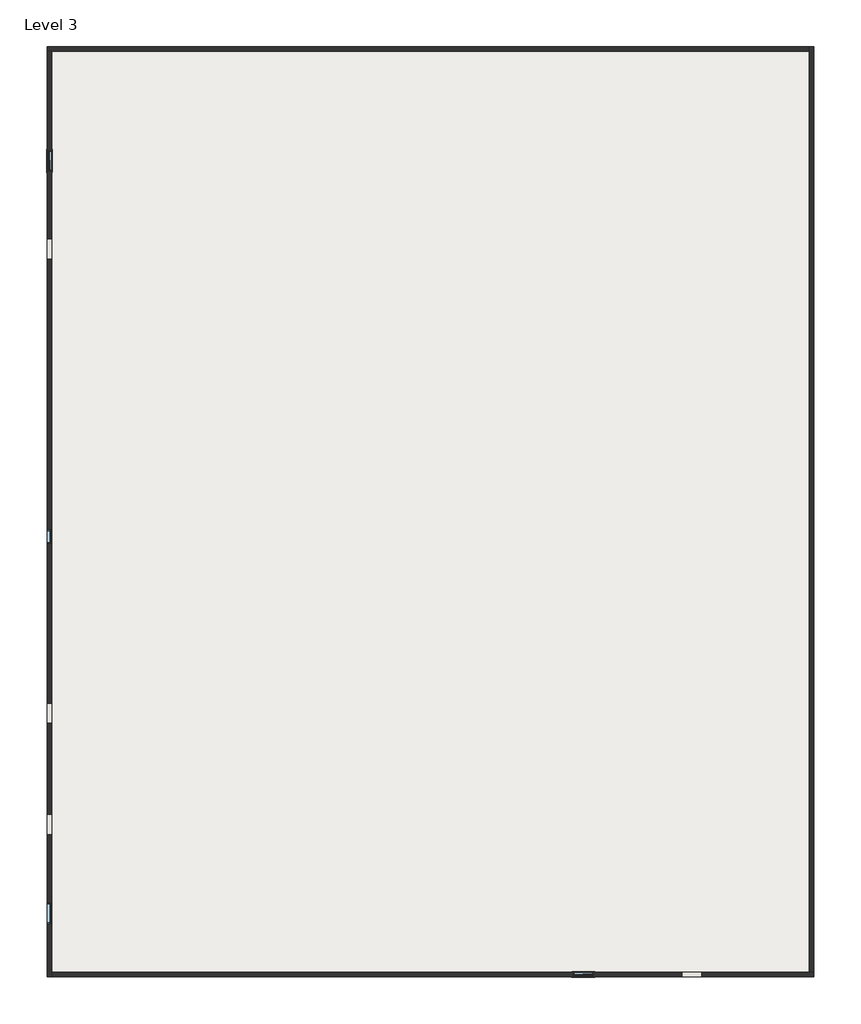
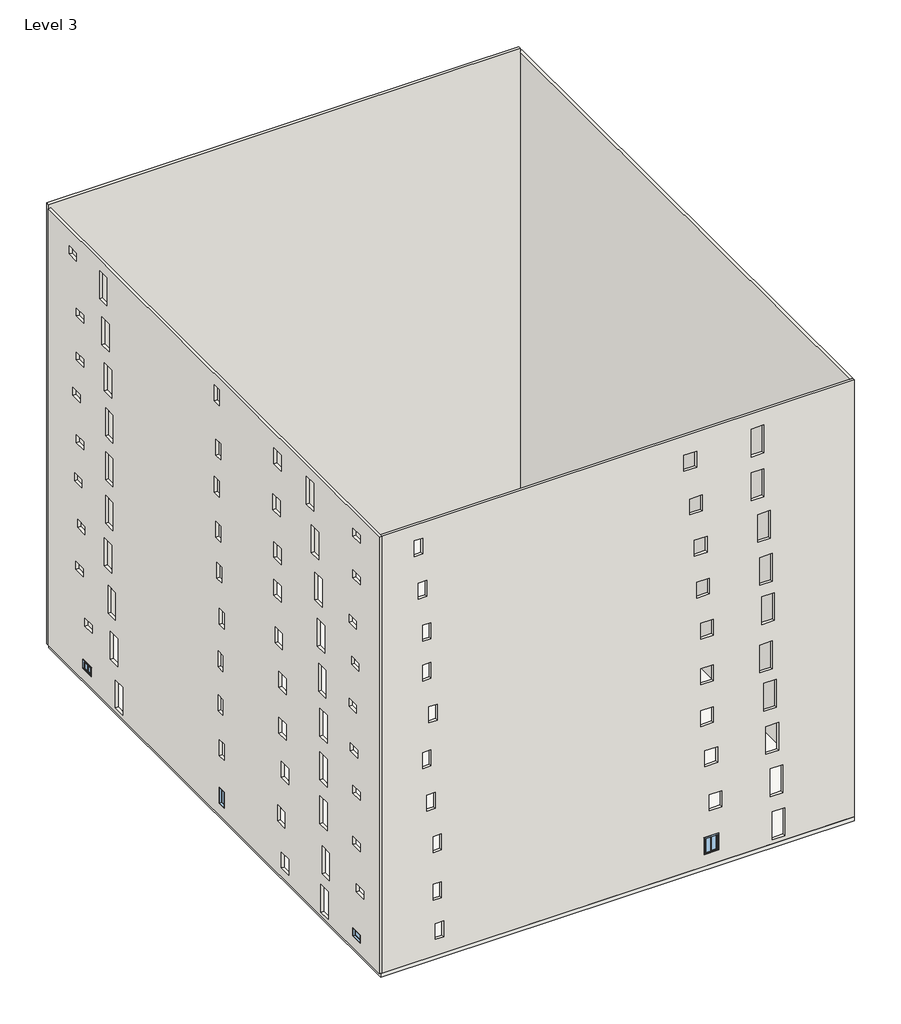
# One storey: 4 walls, 4 windows, 1 slab.
"""IFC4 building model written with IfcOpenShell, lengths in millimetres."""

from ifc_helpers import new_model, si_unit, frame, origin, place, context, project, spatial, polyline, outline, extrude, faceted_brep, transform, mapped, element, save
from components import window_80bd9af0, window_57c3ee1c, window_a4355bb3, window_54100e87

model = new_model("IFC4")

# Units and contexts
model_context = context("Model", 3, world=origin())
ifc_project = project(units=[si_unit("LENGTHUNIT", "METRE", prefix="MILLI")], contexts=[model_context])

# Site, building, storey
site = spatial("IfcSite", under=ifc_project)
building = spatial("IfcBuilding", under=site)
storey = spatial("IfcBuildingStorey", under=building, Name="Level 3", Elevation=6096.0)

# Slab
placement = place(None, origin())
element("IfcSlab", 1, ObjectType="Generic - 12\"", at=placement, inside=storey, context=model_context, shape_type="SweptSolid", body=[
    extrude(outline(polyline([(19165.761926, 20810.2014639), (19165.761926, -20845.7985361), (-15175.038074, -20845.7985361), (-15175.038074, 20810.2014639), (19165.761926, 20810.2014639)])), frame((0.0, 0.0, 5791.2), z_axis=(0.0, 0.0, 1.0), x_axis=(1.0, 0.0, 0.0)), (0.0, 0.0, 1.0), 304.8),
])

# Walls
element("IfcWall", 2, ObjectType="Generic - 8\"", at=placement, inside=storey, context=model_context, shape_type="Brep", body=[
    faceted_brep([(-15276.638074, 20708.6014639, 6096.0), (-15073.438074, 20708.6014639, 6096.0), (18962.561926, 20708.6014639, 6096.0), (18962.561926, 20708.6014639, 39865.082979), (-15276.638074, 20708.6014639, 39865.082979), (-15276.638074, 20708.6014639, 39560.282979), (-15276.638074, 20911.8014639, 6096.0), (-15276.638074, 20911.8014639, 39865.082979), (18962.561926, 20911.8014639, 39865.082979), (18962.561926, 20911.8014639, 39560.282979), (18962.561926, 20911.8014639, 6096.0)], [[[0, 1, 2, 3, 4, 5]], [[6, 7, 8, 9, 10]], [[2, 1, 0, 6, 10]], [[4, 3, 8, 7]], [[0, 5, 4, 7, 6]], [[3, 2, 10, 9, 8]]]),
])
element("IfcWall", 3, ObjectType="Generic - 8\"", at=placement, inside=storey, context=model_context, shape_type="Brep", body=[
    faceted_brep([(-15073.438074, -20845.7985361, 6096.0), (-15073.438074, -20642.5985361, 6096.0), (-15073.438074, 20708.6014639, 6096.0), (-15073.438074, 20708.6014639, 39560.282979), (-15073.438074, -20642.5985361, 39560.282979), (-15073.438074, -20845.7985361, 39560.282979), (-15073.438074, 13342.6014639, 36576.0), (-15073.438074, 13342.6014639, 38709.6), (-15073.438074, 14257.0014639, 38709.6), (-15073.438074, 14257.0014639, 36576.0), (-15073.438074, 13037.8014639, 33223.2), (-15073.438074, 13037.8014639, 35356.8), (-15073.438074, 13952.2014639, 35356.8), (-15073.438074, 13952.2014639, 33223.2), (-15073.438074, 12733.0014639, 29870.4), (-15073.438074, 12733.0014639, 32004.0), (-15073.438074, 13647.4014639, 32004.0), (-15073.438074, 13647.4014639, 29870.4), (-15073.438074, 12580.6014639, 26517.6), (-15073.438074, 12580.6014639, 28651.2), (-15073.438074, 13495.0014639, 28651.2), (-15073.438074, 13495.0014639, 26517.6), (-15073.438074, 12580.6014639, 23164.8), (-15073.438074, 12580.6014639, 25298.4), (-15073.438074, 13495.0014639, 25298.4), (-15073.438074, 13495.0014639, 23164.8), (-15073.438074, 12580.6014639, 19812.0), (-15073.438074, 12580.6014639, 21945.6), (-15073.438074, 13495.0014639, 21945.6), (-15073.438074, 13495.0014639, 19812.0), (-15073.438074, 12733.0014639, 16459.2), (-15073.438074, 12733.0014639, 18592.8), (-15073.438074, 13647.4014639, 18592.8), (-15073.438074, 13647.4014639, 16459.2), (-15073.438074, 12275.8014639, 13106.4), (-15073.438074, 12275.8014639, 15240.0), (-15073.438074, 13190.2014639, 15240.0), (-15073.438074, 13190.2014639, 13106.4), (-15073.438074, 11971.0014639, 9753.6), (-15073.438074, 11971.0014639, 11887.2), (-15073.438074, 12885.4014639, 11887.2), (-15073.438074, 12885.4014639, 9753.6), (-15073.438074, 11361.4014639, 6400.8), (-15073.438074, 11361.4014639, 8534.4), (-15073.438074, 12275.8014639, 8534.4), (-15073.438074, 12275.8014639, 6400.8), (-15073.438074, -12633.3915889, 36576.0), (-15073.438074, -12633.3915889, 38709.6), (-15073.438074, -11718.9915889, 38709.6), (-15073.438074, -11718.9915889, 36576.0), (-15073.438074, -13242.9915889, 33223.2), (-15073.438074, -13242.9915889, 35356.8), (-15073.438074, -12328.5915889, 35356.8), (-15073.438074, -12328.5915889, 33223.2), (-15073.438074, -13700.1915889, 29870.4), (-15073.438074, -13700.1915889, 32004.0), (-15073.438074, -12785.7915889, 32004.0), (-15073.438074, -12785.7915889, 29870.4), (-15073.438074, -14004.9915889, 26517.6), (-15073.438074, -14004.9915889, 28651.2), (-15073.438074, -13090.5915889, 28651.2), (-15073.438074, -13090.5915889, 26517.6), (-15073.438074, -14157.3915889, 23164.8), (-15073.438074, -14157.3915889, 25298.4), (-15073.438074, -13242.9915889, 25298.4), (-15073.438074, -13242.9915889, 23164.8), (-15073.438074, -14309.7915889, 19812.0), (-15073.438074, -14309.7915889, 21945.6), (-15073.438074, -13395.3915889, 21945.6), (-15073.438074, -13395.3915889, 19812.0), (-15073.438074, -14309.7915889, 16459.2), (-15073.438074, -14309.7915889, 18592.8), (-15073.438074, -13395.3915889, 18592.8), (-15073.438074, -13395.3915889, 16459.2), (-15073.438074, -14309.7915889, 13106.4), (-15073.438074, -14309.7915889, 15240.0), (-15073.438074, -13395.3915889, 15240.0), (-15073.438074, -13395.3915889, 13106.4), (-15073.438074, -14462.1915889, 6400.8), (-15073.438074, -14462.1915889, 8534.4), (-15073.438074, -13547.7915889, 8534.4), (-15073.438074, -13547.7915889, 6400.8), (-15073.438074, -14614.5915889, 9448.8), (-15073.438074, -14614.5915889, 11582.4), (-15073.438074, -13700.1915889, 11582.4), (-15073.438074, -13700.1915889, 9448.8), (-15073.438074, -7643.2213044, 38404.8), (-15073.438074, -7643.2213044, 37185.6), (-15073.438074, -8557.6213044, 37185.6), (-15073.438074, -8557.6213044, 38404.8), (-15073.438074, -7490.8213044, 34807.3666062), (-15073.438074, -7490.8213044, 33588.1666062), (-15073.438074, -8405.2213044, 33588.1666062), (-15073.438074, -8405.2213044, 34807.3666062), (-15073.438074, -7617.8213044, 31211.5058376), (-15073.438074, -7617.8213044, 29992.3058376), (-15073.438074, -8532.2213044, 29992.3058376), (-15073.438074, -8532.2213044, 31211.5058376), (-15073.438074, -7643.2213044, 28346.4), (-15073.438074, -7643.2213044, 27127.2), (-15073.438074, -8557.6213044, 27127.2), (-15073.438074, -8557.6213044, 28346.4), (-15073.438074, -7795.6213044, 24794.8201055), (-15073.438074, -7795.6213044, 23575.6201055), (-15073.438074, -8710.0213044, 23575.6201055), (-15073.438074, -8710.0213044, 24794.8201055), (-15073.438074, -8252.8213044, 21640.8), (-15073.438074, -8252.8213044, 20421.6), (-15073.438074, -9167.2213044, 20421.6), (-15073.438074, -9167.2213044, 21640.8), (-15073.438074, -8252.8213044, 18137.3013379), (-15073.438074, -8252.8213044, 16918.1013379), (-15073.438074, -9167.2213044, 16918.1013379), (-15073.438074, -9167.2213044, 18137.3013379), (-15073.438074, -8557.6213044, 14935.2), (-15073.438074, -8557.6213044, 13716.0), (-15073.438074, -9472.0213044, 13716.0), (-15073.438074, -9472.0213044, 14935.2), (-15073.438074, -8100.4213044, 11325.7414578), (-15073.438074, -8100.4213044, 10106.5414578), (-15073.438074, -9014.8213044, 10106.5414578), (-15073.438074, -9014.8213044, 11325.7414578), (-15073.438074, -8557.6213044, 7986.372861), (-15073.438074, -8557.6213044, 6767.172861), (-15073.438074, -9472.0213044, 6767.172861), (-15073.438074, -9472.0213044, 7986.372861), (-15073.438074, -785.2213044, 38709.6), (-15073.438074, -175.6213044, 38709.6), (-15073.438074, -175.6213044, 37490.4), (-15073.438074, -785.2213044, 37490.4), (-15073.438074, -937.6213044, 34644.418592), (-15073.438074, -328.0213044, 34644.418592), (-15073.438074, -328.0213044, 33425.218592), (-15073.438074, -937.6213044, 33425.218592), (-15073.438074, -785.2213044, 31699.2), (-15073.438074, -175.6213044, 31699.2), (-15073.438074, -175.6213044, 30480.0), (-15073.438074, -785.2213044, 30480.0), (-15073.438074, -937.6213044, 28346.4), (-15073.438074, -328.0213044, 28346.4), (-15073.438074, -328.0213044, 27127.2), (-15073.438074, -937.6213044, 27127.2), (-15073.438074, -1090.0213044, 25298.4), (-15073.438074, -480.4213044, 25298.4), (-15073.438074, -480.4213044, 24079.2), (-15073.438074, -1090.0213044, 24079.2), (-15073.438074, -1394.8213044, 21945.6), (-15073.438074, -785.2213044, 21945.6), (-15073.438074, -785.2213044, 20726.4), (-15073.438074, -1394.8213044, 20726.4), (-15073.438074, -1242.4213044, 18592.8), (-15073.438074, -632.8213044, 18592.8), (-15073.438074, -632.8213044, 17373.6), (-15073.438074, -1242.4213044, 17373.6), (-15073.438074, -1242.4213044, 15240.0), (-15073.438074, -632.8213044, 15240.0), (-15073.438074, -632.8213044, 14020.8), (-15073.438074, -1242.4213044, 14020.8), (-15073.438074, -1394.8213044, 11887.2), (-15073.438074, -785.2213044, 11887.2), (-15073.438074, -785.2213044, 10668.0), (-15073.438074, -1394.8213044, 10668.0), (-15073.438074, -1394.8213044, 8229.6), (-15073.438074, -785.2213044, 8229.6), (-15073.438074, -785.2213044, 7010.4), (-15073.438074, -1394.8213044, 7010.4), (-15073.438074, 18067.0014639, 38292.0078244), (-15073.438074, 18067.0014639, 37682.4078244), (-15073.438074, 17152.6014639, 37682.4078244), (-15073.438074, 17152.6014639, 38292.0078244), (-15073.438074, 17152.6014639, 34092.765286), (-15073.438074, 17152.6014639, 33483.165286), (-15073.438074, 16238.2014639, 33483.165286), (-15073.438074, 16238.2014639, 34092.765286), (-15073.438074, 17152.6014639, 30718.6975007), (-15073.438074, 17152.6014639, 30109.0975007), (-15073.438074, 16238.2014639, 30109.0975007), (-15073.438074, 16238.2014639, 30718.6975007), (-15073.438074, 17609.8014639, 27736.8), (-15073.438074, 17609.8014639, 27127.2), (-15073.438074, 16695.4014639, 27127.2), (-15073.438074, 16695.4014639, 27736.8), (-15073.438074, 17152.6014639, 24384.0), (-15073.438074, 17152.6014639, 23774.4), (-15073.438074, 16238.2014639, 23774.4), (-15073.438074, 16238.2014639, 24384.0), (-15073.438074, 17381.2014639, 21336.0), (-15073.438074, 17381.2014639, 20726.4), (-15073.438074, 16466.8014639, 20726.4), (-15073.438074, 16466.8014639, 21336.0), (-15073.438074, 17000.2014639, 17983.2), (-15073.438074, 17000.2014639, 17373.6), (-15073.438074, 16085.8014639, 17373.6), (-15073.438074, 16085.8014639, 17983.2), (-15073.438074, 17228.8014639, 14630.4), (-15073.438074, 17228.8014639, 14020.8), (-15073.438074, 16314.4014639, 14020.8), (-15073.438074, 16314.4014639, 14630.4), (-15073.438074, 16085.8014639, 10972.8), (-15073.438074, 16085.8014639, 10363.2), (-15073.438074, 15171.4014639, 10363.2), (-15073.438074, 15171.4014639, 10972.8), (-15073.438074, 16238.2014639, 7620.0), (-15073.438074, 16238.2014639, 7010.4), (-15073.438074, 15323.8014639, 7010.4), (-15073.438074, 15323.8014639, 7620.0), (-15073.438074, -18460.9099202, 38259.9868241), (-15073.438074, -17546.5099202, 38259.9868241), (-15073.438074, -17546.5099202, 37650.3868241), (-15073.438074, -18460.9099202, 37650.3868241), (-15073.438074, -18460.9099202, 35069.665757), (-15073.438074, -17546.5099202, 35069.665757), (-15073.438074, -17546.5099202, 34460.065757), (-15073.438074, -18460.9099202, 34460.065757), (-15073.438074, -18006.4213044, 31394.4), (-15073.438074, -17092.0213044, 31394.4), (-15073.438074, -17092.0213044, 30784.8), (-15073.438074, -18006.4213044, 30784.8), (-15073.438074, -18311.2213044, 28348.6132762), (-15073.438074, -17396.8213044, 28348.6132762), (-15073.438074, -17396.8213044, 27739.0132762), (-15073.438074, -18311.2213044, 27739.0132762), (-15073.438074, -18006.4213044, 24953.0717638), (-15073.438074, -17092.0213044, 24953.0717638), (-15073.438074, -17092.0213044, 24343.4717638), (-15073.438074, -18006.4213044, 24343.4717638), (-15073.438074, -18158.8213044, 21626.4980928), (-15073.438074, -17244.4213044, 21626.4980928), (-15073.438074, -17244.4213044, 21016.8980928), (-15073.438074, -18158.8213044, 21016.8980928), (-15073.438074, -18460.9099202, 18571.6304295), (-15073.438074, -17546.5099202, 18571.6304295), (-15073.438074, -17546.5099202, 17962.0304295), (-15073.438074, -18460.9099202, 17962.0304295), (-15073.438074, -18460.9099202, 14630.4), (-15073.438074, -17546.5099202, 14630.4), (-15073.438074, -17546.5099202, 14020.8), (-15073.438074, -18460.9099202, 14020.8), (-15073.438074, -18915.3985361, 11277.6), (-15073.438074, -18000.9985361, 11277.6), (-15073.438074, -18000.9985361, 10668.0), (-15073.438074, -18915.3985361, 10668.0), (-15073.438074, -18460.9099202, 7620.0), (-15073.438074, -17546.5099202, 7620.0), (-15073.438074, -17546.5099202, 7010.4), (-15073.438074, -18460.9099202, 7010.4), (-15276.638074, -20845.7985361, 6096.0), (-15276.638074, -20845.7985361, 39560.282979), (-15276.638074, 20708.6014639, 39560.282979), (-15276.638074, 20708.6014639, 6096.0), (-15276.638074, 13342.6014639, 36576.0), (-15276.638074, 14257.0014639, 36576.0), (-15276.638074, 14257.0014639, 38709.6), (-15276.638074, 13342.6014639, 38709.6), (-15276.638074, 13037.8014639, 33223.2), (-15276.638074, 13952.2014639, 33223.2), (-15276.638074, 13952.2014639, 35356.8), (-15276.638074, 13037.8014639, 35356.8), (-15276.638074, 12733.0014639, 29870.4), (-15276.638074, 13647.4014639, 29870.4), (-15276.638074, 13647.4014639, 32004.0), (-15276.638074, 12733.0014639, 32004.0), (-15276.638074, 12580.6014639, 26517.6), (-15276.638074, 13495.0014639, 26517.6), (-15276.638074, 13495.0014639, 28651.2), (-15276.638074, 12580.6014639, 28651.2), (-15276.638074, 12580.6014639, 23164.8), (-15276.638074, 13495.0014639, 23164.8), (-15276.638074, 13495.0014639, 25298.4), (-15276.638074, 12580.6014639, 25298.4), (-15276.638074, 12580.6014639, 19812.0), (-15276.638074, 13495.0014639, 19812.0), (-15276.638074, 13495.0014639, 21945.6), (-15276.638074, 12580.6014639, 21945.6), (-15276.638074, 12733.0014639, 16459.2), (-15276.638074, 13647.4014639, 16459.2), (-15276.638074, 13647.4014639, 18592.8), (-15276.638074, 12733.0014639, 18592.8), (-15276.638074, 12275.8014639, 13106.4), (-15276.638074, 13190.2014639, 13106.4), (-15276.638074, 13190.2014639, 15240.0), (-15276.638074, 12275.8014639, 15240.0), (-15276.638074, 11971.0014639, 9753.6), (-15276.638074, 12885.4014639, 9753.6), (-15276.638074, 12885.4014639, 11887.2), (-15276.638074, 11971.0014639, 11887.2), (-15276.638074, 11361.4014639, 6400.8), (-15276.638074, 12275.8014639, 6400.8), (-15276.638074, 12275.8014639, 8534.4), (-15276.638074, 11361.4014639, 8534.4), (-15276.638074, -12633.3915889, 36576.0), (-15276.638074, -11718.9915889, 36576.0), (-15276.638074, -11718.9915889, 38709.6), (-15276.638074, -12633.3915889, 38709.6), (-15276.638074, -13242.9915889, 33223.2), (-15276.638074, -12328.5915889, 33223.2), (-15276.638074, -12328.5915889, 35356.8), (-15276.638074, -13242.9915889, 35356.8), (-15276.638074, -13700.1915889, 29870.4), (-15276.638074, -12785.7915889, 29870.4), (-15276.638074, -12785.7915889, 32004.0), (-15276.638074, -13700.1915889, 32004.0), (-15276.638074, -14004.9915889, 26517.6), (-15276.638074, -13090.5915889, 26517.6), (-15276.638074, -13090.5915889, 28651.2), (-15276.638074, -14004.9915889, 28651.2), (-15276.638074, -14157.3915889, 23164.8), (-15276.638074, -13242.9915889, 23164.8), (-15276.638074, -13242.9915889, 25298.4), (-15276.638074, -14157.3915889, 25298.4), (-15276.638074, -14309.7915889, 19812.0), (-15276.638074, -13395.3915889, 19812.0), (-15276.638074, -13395.3915889, 21945.6), (-15276.638074, -14309.7915889, 21945.6), (-15276.638074, -14309.7915889, 16459.2), (-15276.638074, -13395.3915889, 16459.2), (-15276.638074, -13395.3915889, 18592.8), (-15276.638074, -14309.7915889, 18592.8), (-15276.638074, -14309.7915889, 13106.4), (-15276.638074, -13395.3915889, 13106.4), (-15276.638074, -13395.3915889, 15240.0), (-15276.638074, -14309.7915889, 15240.0), (-15276.638074, -14462.1915889, 6400.8), (-15276.638074, -13547.7915889, 6400.8), (-15276.638074, -13547.7915889, 8534.4), (-15276.638074, -14462.1915889, 8534.4), (-15276.638074, -14614.5915889, 9448.8), (-15276.638074, -13700.1915889, 9448.8), (-15276.638074, -13700.1915889, 11582.4), (-15276.638074, -14614.5915889, 11582.4), (-15276.638074, -7643.2213044, 38404.8), (-15276.638074, -8557.6213044, 38404.8), (-15276.638074, -8557.6213044, 37185.6), (-15276.638074, -7643.2213044, 37185.6), (-15276.638074, -7490.8213044, 34807.3666062), (-15276.638074, -8405.2213044, 34807.3666062), (-15276.638074, -8405.2213044, 33588.1666062), (-15276.638074, -7490.8213044, 33588.1666062), (-15276.638074, -7617.8213044, 31211.5058376), (-15276.638074, -8532.2213044, 31211.5058376), (-15276.638074, -8532.2213044, 29992.3058376), (-15276.638074, -7617.8213044, 29992.3058376), (-15276.638074, -7643.2213044, 28346.4), (-15276.638074, -8557.6213044, 28346.4), (-15276.638074, -8557.6213044, 27127.2), (-15276.638074, -7643.2213044, 27127.2), (-15276.638074, -7795.6213044, 24794.8201055), (-15276.638074, -8710.0213044, 24794.8201055), (-15276.638074, -8710.0213044, 23575.6201055), (-15276.638074, -7795.6213044, 23575.6201055), (-15276.638074, -8252.8213044, 21640.8), (-15276.638074, -9167.2213044, 21640.8), (-15276.638074, -9167.2213044, 20421.6), (-15276.638074, -8252.8213044, 20421.6), (-15276.638074, -8252.8213044, 18137.3013379), (-15276.638074, -9167.2213044, 18137.3013379), (-15276.638074, -9167.2213044, 16918.1013379), (-15276.638074, -8252.8213044, 16918.1013379), (-15276.638074, -8557.6213044, 14935.2), (-15276.638074, -9472.0213044, 14935.2), (-15276.638074, -9472.0213044, 13716.0), (-15276.638074, -8557.6213044, 13716.0), (-15276.638074, -8100.4213044, 11325.7414578), (-15276.638074, -9014.8213044, 11325.7414578), (-15276.638074, -9014.8213044, 10106.5414578), (-15276.638074, -8100.4213044, 10106.5414578), (-15276.638074, -8557.6213044, 7986.372861), (-15276.638074, -9472.0213044, 7986.372861), (-15276.638074, -9472.0213044, 6767.172861), (-15276.638074, -8557.6213044, 6767.172861), (-15276.638074, -785.2213044, 38709.6), (-15276.638074, -785.2213044, 37490.4), (-15276.638074, -175.6213044, 37490.4), (-15276.638074, -175.6213044, 38709.6), (-15276.638074, -937.6213044, 34644.418592), (-15276.638074, -937.6213044, 33425.218592), (-15276.638074, -328.0213044, 33425.218592), (-15276.638074, -328.0213044, 34644.418592), (-15276.638074, -785.2213044, 31699.2), (-15276.638074, -785.2213044, 30480.0), (-15276.638074, -175.6213044, 30480.0), (-15276.638074, -175.6213044, 31699.2), (-15276.638074, -937.6213044, 28346.4), (-15276.638074, -937.6213044, 27127.2), (-15276.638074, -328.0213044, 27127.2), (-15276.638074, -328.0213044, 28346.4), (-15276.638074, -1090.0213044, 25298.4), (-15276.638074, -1090.0213044, 24079.2), (-15276.638074, -480.4213044, 24079.2), (-15276.638074, -480.4213044, 25298.4), (-15276.638074, -1394.8213044, 21945.6), (-15276.638074, -1394.8213044, 20726.4), (-15276.638074, -785.2213044, 20726.4), (-15276.638074, -785.2213044, 21945.6), (-15276.638074, -1242.4213044, 18592.8), (-15276.638074, -1242.4213044, 17373.6), (-15276.638074, -632.8213044, 17373.6), (-15276.638074, -632.8213044, 18592.8), (-15276.638074, -1242.4213044, 15240.0), (-15276.638074, -1242.4213044, 14020.8), (-15276.638074, -632.8213044, 14020.8), (-15276.638074, -632.8213044, 15240.0), (-15276.638074, -1394.8213044, 11887.2), (-15276.638074, -1394.8213044, 10668.0), (-15276.638074, -785.2213044, 10668.0), (-15276.638074, -785.2213044, 11887.2), (-15276.638074, -1394.8213044, 8229.6), (-15276.638074, -1394.8213044, 7010.4), (-15276.638074, -785.2213044, 7010.4), (-15276.638074, -785.2213044, 8229.6), (-15276.638074, 18067.0014639, 38292.0078244), (-15276.638074, 17152.6014639, 38292.0078244), (-15276.638074, 17152.6014639, 37682.4078244), (-15276.638074, 18067.0014639, 37682.4078244), (-15276.638074, 17152.6014639, 34092.765286), (-15276.638074, 16238.2014639, 34092.765286), (-15276.638074, 16238.2014639, 33483.165286), (-15276.638074, 17152.6014639, 33483.165286), (-15276.638074, 17152.6014639, 30718.6975007), (-15276.638074, 16238.2014639, 30718.6975007), (-15276.638074, 16238.2014639, 30109.0975007), (-15276.638074, 17152.6014639, 30109.0975007), (-15276.638074, 17609.8014639, 27736.8), (-15276.638074, 16695.4014639, 27736.8), (-15276.638074, 16695.4014639, 27127.2), (-15276.638074, 17609.8014639, 27127.2), (-15276.638074, 17152.6014639, 24384.0), (-15276.638074, 16238.2014639, 24384.0), (-15276.638074, 16238.2014639, 23774.4), (-15276.638074, 17152.6014639, 23774.4), (-15276.638074, 17381.2014639, 21336.0), (-15276.638074, 16466.8014639, 21336.0), (-15276.638074, 16466.8014639, 20726.4), (-15276.638074, 17381.2014639, 20726.4), (-15276.638074, 17000.2014639, 17983.2), (-15276.638074, 16085.8014639, 17983.2), (-15276.638074, 16085.8014639, 17373.6), (-15276.638074, 17000.2014639, 17373.6), (-15276.638074, 17228.8014639, 14630.4), (-15276.638074, 16314.4014639, 14630.4), (-15276.638074, 16314.4014639, 14020.8), (-15276.638074, 17228.8014639, 14020.8), (-15276.638074, 16085.8014639, 10972.8), (-15276.638074, 15171.4014639, 10972.8), (-15276.638074, 15171.4014639, 10363.2), (-15276.638074, 16085.8014639, 10363.2), (-15276.638074, 16238.2014639, 7620.0), (-15276.638074, 15323.8014639, 7620.0), (-15276.638074, 15323.8014639, 7010.4), (-15276.638074, 16238.2014639, 7010.4), (-15276.638074, -18460.9099202, 38259.9868241), (-15276.638074, -18460.9099202, 37650.3868241), (-15276.638074, -17546.5099202, 37650.3868241), (-15276.638074, -17546.5099202, 38259.9868241), (-15276.638074, -18460.9099202, 35069.665757), (-15276.638074, -18460.9099202, 34460.065757), (-15276.638074, -17546.5099202, 34460.065757), (-15276.638074, -17546.5099202, 35069.665757), (-15276.638074, -18006.4213044, 31394.4), (-15276.638074, -18006.4213044, 30784.8), (-15276.638074, -17092.0213044, 30784.8), (-15276.638074, -17092.0213044, 31394.4), (-15276.638074, -18311.2213044, 28348.6132762), (-15276.638074, -18311.2213044, 27739.0132762), (-15276.638074, -17396.8213044, 27739.0132762), (-15276.638074, -17396.8213044, 28348.6132762), (-15276.638074, -18006.4213044, 24953.0717638), (-15276.638074, -18006.4213044, 24343.4717638), (-15276.638074, -17092.0213044, 24343.4717638), (-15276.638074, -17092.0213044, 24953.0717638), (-15276.638074, -18158.8213044, 21626.4980928), (-15276.638074, -18158.8213044, 21016.8980928), (-15276.638074, -17244.4213044, 21016.8980928), (-15276.638074, -17244.4213044, 21626.4980928), (-15276.638074, -18460.9099202, 18571.6304295), (-15276.638074, -18460.9099202, 17962.0304295), (-15276.638074, -17546.5099202, 17962.0304295), (-15276.638074, -17546.5099202, 18571.6304295), (-15276.638074, -18460.9099202, 14630.4), (-15276.638074, -18460.9099202, 14020.8), (-15276.638074, -17546.5099202, 14020.8), (-15276.638074, -17546.5099202, 14630.4), (-15276.638074, -18915.3985361, 11277.6), (-15276.638074, -18915.3985361, 10668.0), (-15276.638074, -18000.9985361, 10668.0), (-15276.638074, -18000.9985361, 11277.6), (-15276.638074, -18460.9099202, 7620.0), (-15276.638074, -18460.9099202, 7010.4), (-15276.638074, -17546.5099202, 7010.4), (-15276.638074, -17546.5099202, 7620.0)], [[[0, 1, 2, 3, 4, 5], [6, 7, 8, 9], [10, 11, 12, 13], [14, 15, 16, 17], [18, 19, 20, 21], [22, 23, 24, 25], [26, 27, 28, 29], [30, 31, 32, 33], [34, 35, 36, 37], [38, 39, 40, 41], [42, 43, 44, 45], [46, 47, 48, 49], [50, 51, 52, 53], [54, 55, 56, 57], [58, 59, 60, 61], [62, 63, 64, 65], [66, 67, 68, 69], [70, 71, 72, 73], [74, 75, 76, 77], [78, 79, 80, 81], [82, 83, 84, 85], [86, 87, 88, 89], [90, 91, 92, 93], [94, 95, 96, 97], [98, 99, 100, 101], [102, 103, 104, 105], [106, 107, 108, 109], [110, 111, 112, 113], [114, 115, 116, 117], [118, 119, 120, 121], [122, 123, 124, 125], [126, 127, 128, 129], [130, 131, 132, 133], [134, 135, 136, 137], [138, 139, 140, 141], [142, 143, 144, 145], [146, 147, 148, 149], [150, 151, 152, 153], [154, 155, 156, 157], [158, 159, 160, 161], [162, 163, 164, 165], [166, 167, 168, 169], [170, 171, 172, 173], [174, 175, 176, 177], [178, 179, 180, 181], [182, 183, 184, 185], [186, 187, 188, 189], [190, 191, 192, 193], [194, 195, 196, 197], [198, 199, 200, 201], [202, 203, 204, 205], [206, 207, 208, 209], [210, 211, 212, 213], [214, 215, 216, 217], [218, 219, 220, 221], [222, 223, 224, 225], [226, 227, 228, 229], [230, 231, 232, 233], [234, 235, 236, 237], [238, 239, 240, 241], [242, 243, 244, 245]], [[246, 247, 248, 249], [250, 251, 252, 253], [254, 255, 256, 257], [258, 259, 260, 261], [262, 263, 264, 265], [266, 267, 268, 269], [270, 271, 272, 273], [274, 275, 276, 277], [278, 279, 280, 281], [282, 283, 284, 285], [286, 287, 288, 289], [290, 291, 292, 293], [294, 295, 296, 297], [298, 299, 300, 301], [302, 303, 304, 305], [306, 307, 308, 309], [310, 311, 312, 313], [314, 315, 316, 317], [318, 319, 320, 321], [322, 323, 324, 325], [326, 327, 328, 329], [330, 331, 332, 333], [334, 335, 336, 337], [338, 339, 340, 341], [342, 343, 344, 345], [346, 347, 348, 349], [350, 351, 352, 353], [354, 355, 356, 357], [358, 359, 360, 361], [362, 363, 364, 365], [366, 367, 368, 369], [370, 371, 372, 373], [374, 375, 376, 377], [378, 379, 380, 381], [382, 383, 384, 385], [386, 387, 388, 389], [390, 391, 392, 393], [394, 395, 396, 397], [398, 399, 400, 401], [402, 403, 404, 405], [406, 407, 408, 409], [410, 411, 412, 413], [414, 415, 416, 417], [418, 419, 420, 421], [422, 423, 424, 425], [426, 427, 428, 429], [430, 431, 432, 433], [434, 435, 436, 437], [438, 439, 440, 441], [442, 443, 444, 445], [446, 447, 448, 449], [450, 451, 452, 453], [454, 455, 456, 457], [458, 459, 460, 461], [462, 463, 464, 465], [466, 467, 468, 469], [470, 471, 472, 473], [474, 475, 476, 477], [478, 479, 480, 481], [482, 483, 484, 485], [486, 487, 488, 489]], [[2, 1, 0, 246, 249]], [[5, 4, 3, 248, 247]], [[0, 5, 247, 246]], [[3, 2, 249, 248]], [[251, 250, 6, 9]], [[252, 251, 9, 8]], [[253, 252, 8, 7]], [[250, 253, 7, 6]], [[255, 254, 10, 13]], [[256, 255, 13, 12]], [[257, 256, 12, 11]], [[254, 257, 11, 10]], [[259, 258, 14, 17]], [[260, 259, 17, 16]], [[261, 260, 16, 15]], [[258, 261, 15, 14]], [[263, 262, 18, 21]], [[264, 263, 21, 20]], [[265, 264, 20, 19]], [[262, 265, 19, 18]], [[267, 266, 22, 25]], [[268, 267, 25, 24]], [[269, 268, 24, 23]], [[266, 269, 23, 22]], [[271, 270, 26, 29]], [[272, 271, 29, 28]], [[273, 272, 28, 27]], [[270, 273, 27, 26]], [[275, 274, 30, 33]], [[276, 275, 33, 32]], [[277, 276, 32, 31]], [[274, 277, 31, 30]], [[279, 278, 34, 37]], [[280, 279, 37, 36]], [[281, 280, 36, 35]], [[278, 281, 35, 34]], [[283, 282, 38, 41]], [[284, 283, 41, 40]], [[285, 284, 40, 39]], [[282, 285, 39, 38]], [[287, 286, 42, 45]], [[288, 287, 45, 44]], [[289, 288, 44, 43]], [[286, 289, 43, 42]], [[291, 290, 46, 49]], [[292, 291, 49, 48]], [[293, 292, 48, 47]], [[290, 293, 47, 46]], [[295, 294, 50, 53]], [[296, 295, 53, 52]], [[297, 296, 52, 51]], [[294, 297, 51, 50]], [[299, 298, 54, 57]], [[300, 299, 57, 56]], [[301, 300, 56, 55]], [[298, 301, 55, 54]], [[303, 302, 58, 61]], [[304, 303, 61, 60]], [[305, 304, 60, 59]], [[302, 305, 59, 58]], [[307, 306, 62, 65]], [[308, 307, 65, 64]], [[309, 308, 64, 63]], [[306, 309, 63, 62]], [[311, 310, 66, 69]], [[312, 311, 69, 68]], [[313, 312, 68, 67]], [[310, 313, 67, 66]], [[315, 314, 70, 73]], [[316, 315, 73, 72]], [[317, 316, 72, 71]], [[314, 317, 71, 70]], [[319, 318, 74, 77]], [[320, 319, 77, 76]], [[321, 320, 76, 75]], [[318, 321, 75, 74]], [[323, 322, 78, 81]], [[324, 323, 81, 80]], [[325, 324, 80, 79]], [[322, 325, 79, 78]], [[327, 326, 82, 85]], [[328, 327, 85, 84]], [[329, 328, 84, 83]], [[326, 329, 83, 82]], [[87, 86, 330, 333]], [[88, 87, 333, 332]], [[89, 88, 332, 331]], [[86, 89, 331, 330]], [[91, 90, 334, 337]], [[92, 91, 337, 336]], [[93, 92, 336, 335]], [[90, 93, 335, 334]], [[95, 94, 338, 341]], [[96, 95, 341, 340]], [[97, 96, 340, 339]], [[94, 97, 339, 338]], [[99, 98, 342, 345]], [[100, 99, 345, 344]], [[101, 100, 344, 343]], [[98, 101, 343, 342]], [[103, 102, 346, 349]], [[104, 103, 349, 348]], [[105, 104, 348, 347]], [[102, 105, 347, 346]], [[107, 106, 350, 353]], [[108, 107, 353, 352]], [[109, 108, 352, 351]], [[106, 109, 351, 350]], [[111, 110, 354, 357]], [[112, 111, 357, 356]], [[113, 112, 356, 355]], [[110, 113, 355, 354]], [[115, 114, 358, 361]], [[116, 115, 361, 360]], [[117, 116, 360, 359]], [[114, 117, 359, 358]], [[119, 118, 362, 365]], [[120, 119, 365, 364]], [[121, 120, 364, 363]], [[118, 121, 363, 362]], [[123, 122, 366, 369]], [[124, 123, 369, 368]], [[125, 124, 368, 367]], [[122, 125, 367, 366]], [[371, 370, 126, 129]], [[372, 371, 129, 128]], [[373, 372, 128, 127]], [[370, 373, 127, 126]], [[375, 374, 130, 133]], [[376, 375, 133, 132]], [[377, 376, 132, 131]], [[374, 377, 131, 130]], [[379, 378, 134, 137]], [[380, 379, 137, 136]], [[381, 380, 136, 135]], [[378, 381, 135, 134]], [[383, 382, 138, 141]], [[384, 383, 141, 140]], [[385, 384, 140, 139]], [[382, 385, 139, 138]], [[387, 386, 142, 145]], [[388, 387, 145, 144]], [[389, 388, 144, 143]], [[386, 389, 143, 142]], [[391, 390, 146, 149]], [[392, 391, 149, 148]], [[393, 392, 148, 147]], [[390, 393, 147, 146]], [[395, 394, 150, 153]], [[396, 395, 153, 152]], [[397, 396, 152, 151]], [[394, 397, 151, 150]], [[399, 398, 154, 157]], [[400, 399, 157, 156]], [[401, 400, 156, 155]], [[398, 401, 155, 154]], [[403, 402, 158, 161]], [[404, 403, 161, 160]], [[405, 404, 160, 159]], [[402, 405, 159, 158]], [[407, 406, 162, 165]], [[408, 407, 165, 164]], [[409, 408, 164, 163]], [[406, 409, 163, 162]], [[167, 166, 410, 413]], [[168, 167, 413, 412]], [[169, 168, 412, 411]], [[166, 169, 411, 410]], [[171, 170, 414, 417]], [[172, 171, 417, 416]], [[173, 172, 416, 415]], [[170, 173, 415, 414]], [[175, 174, 418, 421]], [[176, 175, 421, 420]], [[177, 176, 420, 419]], [[174, 177, 419, 418]], [[179, 178, 422, 425]], [[180, 179, 425, 424]], [[181, 180, 424, 423]], [[178, 181, 423, 422]], [[183, 182, 426, 429]], [[184, 183, 429, 428]], [[185, 184, 428, 427]], [[182, 185, 427, 426]], [[187, 186, 430, 433]], [[188, 187, 433, 432]], [[189, 188, 432, 431]], [[186, 189, 431, 430]], [[191, 190, 434, 437]], [[192, 191, 437, 436]], [[193, 192, 436, 435]], [[190, 193, 435, 434]], [[195, 194, 438, 441]], [[196, 195, 441, 440]], [[197, 196, 440, 439]], [[194, 197, 439, 438]], [[199, 198, 442, 445]], [[200, 199, 445, 444]], [[201, 200, 444, 443]], [[198, 201, 443, 442]], [[203, 202, 446, 449]], [[204, 203, 449, 448]], [[205, 204, 448, 447]], [[202, 205, 447, 446]], [[451, 450, 206, 209]], [[452, 451, 209, 208]], [[453, 452, 208, 207]], [[450, 453, 207, 206]], [[455, 454, 210, 213]], [[456, 455, 213, 212]], [[457, 456, 212, 211]], [[454, 457, 211, 210]], [[459, 458, 214, 217]], [[460, 459, 217, 216]], [[461, 460, 216, 215]], [[458, 461, 215, 214]], [[463, 462, 218, 221]], [[464, 463, 221, 220]], [[465, 464, 220, 219]], [[462, 465, 219, 218]], [[467, 466, 222, 225]], [[468, 467, 225, 224]], [[469, 468, 224, 223]], [[466, 469, 223, 222]], [[471, 470, 226, 229]], [[472, 471, 229, 228]], [[473, 472, 228, 227]], [[470, 473, 227, 226]], [[475, 474, 230, 233]], [[476, 475, 233, 232]], [[477, 476, 232, 231]], [[474, 477, 231, 230]], [[479, 478, 234, 237]], [[480, 479, 237, 236]], [[481, 480, 236, 235]], [[478, 481, 235, 234]], [[483, 482, 238, 241]], [[484, 483, 241, 240]], [[485, 484, 240, 239]], [[482, 485, 239, 238]], [[487, 486, 242, 245]], [[488, 487, 245, 244]], [[489, 488, 244, 243]], [[486, 489, 243, 242]]]),
])
element("IfcWall", 4, ObjectType="Generic - 8\"", at=placement, inside=storey, context=model_context, shape_type="Brep", body=[
    faceted_brep([(19165.761926, -20642.5985361, 6096.0), (18962.561926, -20642.5985361, 6096.0), (-15073.438074, -20642.5985361, 6096.0), (-15073.438074, -20642.5985361, 39560.282979), (18962.561926, -20642.5985361, 39560.282979), (19165.761926, -20642.5985361, 39560.282979), (11698.161926, -20642.5985361, 36271.2), (12612.561926, -20642.5985361, 36271.2), (12612.561926, -20642.5985361, 38404.8), (11698.161926, -20642.5985361, 38404.8), (11698.161926, -20642.5985361, 32918.4), (12612.561926, -20642.5985361, 32918.4), (12612.561926, -20642.5985361, 35052.0), (11698.161926, -20642.5985361, 35052.0), (12155.361926, -20642.5985361, 29565.6), (13069.761926, -20642.5985361, 29565.6), (13069.761926, -20642.5985361, 31699.2), (12155.361926, -20642.5985361, 31699.2), (12307.761926, -20642.5985361, 26212.8), (13222.161926, -20642.5985361, 26212.8), (13222.161926, -20642.5985361, 28346.4), (12307.761926, -20642.5985361, 28346.4), (12307.761926, -20642.5985361, 19507.2), (13222.161926, -20642.5985361, 19507.2), (13222.161926, -20642.5985361, 21640.8), (12307.761926, -20642.5985361, 21640.8), (12460.161926, -20642.5985361, 23164.8), (13374.561926, -20642.5985361, 23164.8), (13374.561926, -20642.5985361, 25298.4), (12460.161926, -20642.5985361, 25298.4), (12612.561926, -20642.5985361, 16459.2), (13526.961926, -20642.5985361, 16459.2), (13526.961926, -20642.5985361, 18592.8), (12612.561926, -20642.5985361, 18592.8), (12764.961926, -20642.5985361, 13106.4), (13679.361926, -20642.5985361, 13106.4), (13679.361926, -20642.5985361, 15240.0), (12764.961926, -20642.5985361, 15240.0), (13069.761926, -20642.5985361, 9753.6), (13984.161926, -20642.5985361, 9753.6), (13984.161926, -20642.5985361, 11887.2), (13069.761926, -20642.5985361, 11887.2), (13222.161926, -20642.5985361, 6400.8), (14136.561926, -20642.5985361, 6400.8), (14136.561926, -20642.5985361, 8534.4), (13222.161926, -20642.5985361, 8534.4), (-12736.638074, -20642.5985361, 38404.8), (-12736.638074, -20642.5985361, 37185.6), (-12127.038074, -20642.5985361, 37185.6), (-12127.038074, -20642.5985361, 38404.8), (-12431.838074, -20642.5985361, 35052.0), (-12431.838074, -20642.5985361, 33832.8), (-11822.238074, -20642.5985361, 33832.8), (-11822.238074, -20642.5985361, 35052.0), (-12127.038074, -20642.5985361, 31699.2), (-12127.038074, -20642.5985361, 30480.0), (-11517.438074, -20642.5985361, 30480.0), (-11517.438074, -20642.5985361, 31699.2), (-12127.038074, -20642.5985361, 28651.2), (-12127.038074, -20642.5985361, 27432.0), (-11517.438074, -20642.5985361, 27432.0), (-11517.438074, -20642.5985361, 28651.2), (-12127.038074, -20642.5985361, 21945.6), (-12127.038074, -20642.5985361, 20726.4), (-11517.438074, -20642.5985361, 20726.4), (-11517.438074, -20642.5985361, 21945.6), (-11669.838074, -20642.5985361, 25298.4), (-11669.838074, -20642.5985361, 24079.2), (-11060.238074, -20642.5985361, 24079.2), (-11060.238074, -20642.5985361, 25298.4), (-11822.238074, -20642.5985361, 18592.8), (-11822.238074, -20642.5985361, 17373.6), (-11212.638074, -20642.5985361, 17373.6), (-11212.638074, -20642.5985361, 18592.8), (-11365.038074, -20642.5985361, 15240.0), (-11365.038074, -20642.5985361, 14020.8), (-10755.438074, -20642.5985361, 14020.8), (-10755.438074, -20642.5985361, 15240.0), (-11365.038074, -20642.5985361, 11582.4), (-11365.038074, -20642.5985361, 10363.2), (-10755.438074, -20642.5985361, 10363.2), (-10755.438074, -20642.5985361, 11582.4), (-11212.638074, -20642.5985361, 8534.4), (-11212.638074, -20642.5985361, 7315.2), (-10603.038074, -20642.5985361, 7315.2), (-10603.038074, -20642.5985361, 8534.4), (6821.361926, -20642.5985361, 38101.5341516), (6821.361926, -20642.5985361, 36882.3341516), (7735.761926, -20642.5985361, 36882.3341516), (7735.761926, -20642.5985361, 38101.5341516), (7227.761926, -20642.5985361, 34616.5595091), (7227.761926, -20642.5985361, 33397.3595091), (8142.161926, -20642.5985361, 33397.3595091), (8142.161926, -20642.5985361, 34616.5595091), (7583.361926, -20642.5985361, 31327.3828035), (7583.361926, -20642.5985361, 30108.1828035), (8497.761926, -20642.5985361, 30108.1828035), (8497.761926, -20642.5985361, 31327.3828035), (7735.761926, -20642.5985361, 28058.6536631), (7735.761926, -20642.5985361, 26839.4536631), (8650.161926, -20642.5985361, 26839.4536631), (8650.161926, -20642.5985361, 28058.6536631), (8040.561926, -20642.5985361, 24806.7129205), (8040.561926, -20642.5985361, 23587.5129205), (8954.961926, -20642.5985361, 23587.5129205), (8954.961926, -20642.5985361, 24806.7129205), (8040.561926, -20642.5985361, 21313.2342809), (8040.561926, -20642.5985361, 20094.0342809), (8954.961926, -20642.5985361, 20094.0342809), (8954.961926, -20642.5985361, 21313.2342809), (8040.561926, -20642.5985361, 18106.3578988), (8040.561926, -20642.5985361, 16887.1578988), (8954.961926, -20642.5985361, 16887.1578988), (8954.961926, -20642.5985361, 18106.3578988), (8345.361926, -20642.5985361, 14935.2), (8345.361926, -20642.5985361, 13716.0), (9259.761926, -20642.5985361, 13716.0), (9259.761926, -20642.5985361, 14935.2), (8650.161926, -20642.5985361, 11449.3942228), (8650.161926, -20642.5985361, 10230.1942228), (9564.561926, -20642.5985361, 10230.1942228), (9564.561926, -20642.5985361, 11449.3942228), (8345.361926, -20642.5985361, 8229.6), (8345.361926, -20642.5985361, 7010.4), (9259.761926, -20642.5985361, 7010.4), (9259.761926, -20642.5985361, 8229.6), (19165.761926, -20845.7985361, 6096.0), (19165.761926, -20845.7985361, 39560.282979), (-15073.438074, -20845.7985361, 39560.282979), (-15073.438074, -20845.7985361, 6096.0), (11698.161926, -20845.7985361, 36271.2), (11698.161926, -20845.7985361, 38404.8), (12612.561926, -20845.7985361, 38404.8), (12612.561926, -20845.7985361, 36271.2), (11698.161926, -20845.7985361, 32918.4), (11698.161926, -20845.7985361, 35052.0), (12612.561926, -20845.7985361, 35052.0), (12612.561926, -20845.7985361, 32918.4), (12155.361926, -20845.7985361, 29565.6), (12155.361926, -20845.7985361, 31699.2), (13069.761926, -20845.7985361, 31699.2), (13069.761926, -20845.7985361, 29565.6), (12307.761926, -20845.7985361, 26212.8), (12307.761926, -20845.7985361, 28346.4), (13222.161926, -20845.7985361, 28346.4), (13222.161926, -20845.7985361, 26212.8), (12307.761926, -20845.7985361, 19507.2), (12307.761926, -20845.7985361, 21640.8), (13222.161926, -20845.7985361, 21640.8), (13222.161926, -20845.7985361, 19507.2), (12460.161926, -20845.7985361, 23164.8), (12460.161926, -20845.7985361, 25298.4), (13374.561926, -20845.7985361, 25298.4), (13374.561926, -20845.7985361, 23164.8), (12612.561926, -20845.7985361, 16459.2), (12612.561926, -20845.7985361, 18592.8), (13526.961926, -20845.7985361, 18592.8), (13526.961926, -20845.7985361, 16459.2), (12764.961926, -20845.7985361, 13106.4), (12764.961926, -20845.7985361, 15240.0), (13679.361926, -20845.7985361, 15240.0), (13679.361926, -20845.7985361, 13106.4), (13069.761926, -20845.7985361, 9753.6), (13069.761926, -20845.7985361, 11887.2), (13984.161926, -20845.7985361, 11887.2), (13984.161926, -20845.7985361, 9753.6), (13222.161926, -20845.7985361, 6400.8), (13222.161926, -20845.7985361, 8534.4), (14136.561926, -20845.7985361, 8534.4), (14136.561926, -20845.7985361, 6400.8), (-12736.638074, -20845.7985361, 38404.8), (-12127.038074, -20845.7985361, 38404.8), (-12127.038074, -20845.7985361, 37185.6), (-12736.638074, -20845.7985361, 37185.6), (-12431.838074, -20845.7985361, 35052.0), (-11822.238074, -20845.7985361, 35052.0), (-11822.238074, -20845.7985361, 33832.8), (-12431.838074, -20845.7985361, 33832.8), (-12127.038074, -20845.7985361, 31699.2), (-11517.438074, -20845.7985361, 31699.2), (-11517.438074, -20845.7985361, 30480.0), (-12127.038074, -20845.7985361, 30480.0), (-12127.038074, -20845.7985361, 28651.2), (-11517.438074, -20845.7985361, 28651.2), (-11517.438074, -20845.7985361, 27432.0), (-12127.038074, -20845.7985361, 27432.0), (-12127.038074, -20845.7985361, 21945.6), (-11517.438074, -20845.7985361, 21945.6), (-11517.438074, -20845.7985361, 20726.4), (-12127.038074, -20845.7985361, 20726.4), (-11669.838074, -20845.7985361, 25298.4), (-11060.238074, -20845.7985361, 25298.4), (-11060.238074, -20845.7985361, 24079.2), (-11669.838074, -20845.7985361, 24079.2), (-11822.238074, -20845.7985361, 18592.8), (-11212.638074, -20845.7985361, 18592.8), (-11212.638074, -20845.7985361, 17373.6), (-11822.238074, -20845.7985361, 17373.6), (-11365.038074, -20845.7985361, 15240.0), (-10755.438074, -20845.7985361, 15240.0), (-10755.438074, -20845.7985361, 14020.8), (-11365.038074, -20845.7985361, 14020.8), (-11365.038074, -20845.7985361, 11582.4), (-10755.438074, -20845.7985361, 11582.4), (-10755.438074, -20845.7985361, 10363.2), (-11365.038074, -20845.7985361, 10363.2), (-11212.638074, -20845.7985361, 8534.4), (-10603.038074, -20845.7985361, 8534.4), (-10603.038074, -20845.7985361, 7315.2), (-11212.638074, -20845.7985361, 7315.2), (6821.361926, -20845.7985361, 38101.5341516), (7735.761926, -20845.7985361, 38101.5341516), (7735.761926, -20845.7985361, 36882.3341516), (6821.361926, -20845.7985361, 36882.3341516), (7227.761926, -20845.7985361, 34616.5595091), (8142.161926, -20845.7985361, 34616.5595091), (8142.161926, -20845.7985361, 33397.3595091), (7227.761926, -20845.7985361, 33397.3595091), (7583.361926, -20845.7985361, 31327.3828035), (8497.761926, -20845.7985361, 31327.3828035), (8497.761926, -20845.7985361, 30108.1828035), (7583.361926, -20845.7985361, 30108.1828035), (7735.761926, -20845.7985361, 28058.6536631), (8650.161926, -20845.7985361, 28058.6536631), (8650.161926, -20845.7985361, 26839.4536631), (7735.761926, -20845.7985361, 26839.4536631), (8040.561926, -20845.7985361, 24806.7129205), (8954.961926, -20845.7985361, 24806.7129205), (8954.961926, -20845.7985361, 23587.5129205), (8040.561926, -20845.7985361, 23587.5129205), (8040.561926, -20845.7985361, 21313.2342809), (8954.961926, -20845.7985361, 21313.2342809), (8954.961926, -20845.7985361, 20094.0342809), (8040.561926, -20845.7985361, 20094.0342809), (8040.561926, -20845.7985361, 18106.3578988), (8954.961926, -20845.7985361, 18106.3578988), (8954.961926, -20845.7985361, 16887.1578988), (8040.561926, -20845.7985361, 16887.1578988), (8345.361926, -20845.7985361, 14935.2), (9259.761926, -20845.7985361, 14935.2), (9259.761926, -20845.7985361, 13716.0), (8345.361926, -20845.7985361, 13716.0), (8650.161926, -20845.7985361, 11449.3942228), (9564.561926, -20845.7985361, 11449.3942228), (9564.561926, -20845.7985361, 10230.1942228), (8650.161926, -20845.7985361, 10230.1942228), (8345.361926, -20845.7985361, 8229.6), (9259.761926, -20845.7985361, 8229.6), (9259.761926, -20845.7985361, 7010.4), (8345.361926, -20845.7985361, 7010.4)], [[[0, 1, 2, 3, 4, 5], [6, 7, 8, 9], [10, 11, 12, 13], [14, 15, 16, 17], [18, 19, 20, 21], [22, 23, 24, 25], [26, 27, 28, 29], [30, 31, 32, 33], [34, 35, 36, 37], [38, 39, 40, 41], [42, 43, 44, 45], [46, 47, 48, 49], [50, 51, 52, 53], [54, 55, 56, 57], [58, 59, 60, 61], [62, 63, 64, 65], [66, 67, 68, 69], [70, 71, 72, 73], [74, 75, 76, 77], [78, 79, 80, 81], [82, 83, 84, 85], [86, 87, 88, 89], [90, 91, 92, 93], [94, 95, 96, 97], [98, 99, 100, 101], [102, 103, 104, 105], [106, 107, 108, 109], [110, 111, 112, 113], [114, 115, 116, 117], [118, 119, 120, 121], [122, 123, 124, 125]], [[126, 127, 128, 129], [130, 131, 132, 133], [134, 135, 136, 137], [138, 139, 140, 141], [142, 143, 144, 145], [146, 147, 148, 149], [150, 151, 152, 153], [154, 155, 156, 157], [158, 159, 160, 161], [162, 163, 164, 165], [166, 167, 168, 169], [170, 171, 172, 173], [174, 175, 176, 177], [178, 179, 180, 181], [182, 183, 184, 185], [186, 187, 188, 189], [190, 191, 192, 193], [194, 195, 196, 197], [198, 199, 200, 201], [202, 203, 204, 205], [206, 207, 208, 209], [210, 211, 212, 213], [214, 215, 216, 217], [218, 219, 220, 221], [222, 223, 224, 225], [226, 227, 228, 229], [230, 231, 232, 233], [234, 235, 236, 237], [238, 239, 240, 241], [242, 243, 244, 245], [246, 247, 248, 249]], [[2, 1, 0, 126, 129]], [[5, 4, 3, 128, 127]], [[0, 5, 127, 126]], [[3, 2, 129, 128]], [[7, 6, 130, 133]], [[8, 7, 133, 132]], [[9, 8, 132, 131]], [[6, 9, 131, 130]], [[11, 10, 134, 137]], [[12, 11, 137, 136]], [[13, 12, 136, 135]], [[10, 13, 135, 134]], [[15, 14, 138, 141]], [[16, 15, 141, 140]], [[17, 16, 140, 139]], [[14, 17, 139, 138]], [[19, 18, 142, 145]], [[20, 19, 145, 144]], [[21, 20, 144, 143]], [[18, 21, 143, 142]], [[23, 22, 146, 149]], [[24, 23, 149, 148]], [[25, 24, 148, 147]], [[22, 25, 147, 146]], [[27, 26, 150, 153]], [[28, 27, 153, 152]], [[29, 28, 152, 151]], [[26, 29, 151, 150]], [[31, 30, 154, 157]], [[32, 31, 157, 156]], [[33, 32, 156, 155]], [[30, 33, 155, 154]], [[35, 34, 158, 161]], [[36, 35, 161, 160]], [[37, 36, 160, 159]], [[34, 37, 159, 158]], [[39, 38, 162, 165]], [[40, 39, 165, 164]], [[41, 40, 164, 163]], [[38, 41, 163, 162]], [[43, 42, 166, 169]], [[44, 43, 169, 168]], [[45, 44, 168, 167]], [[42, 45, 167, 166]], [[47, 46, 170, 173]], [[48, 47, 173, 172]], [[49, 48, 172, 171]], [[46, 49, 171, 170]], [[51, 50, 174, 177]], [[52, 51, 177, 176]], [[53, 52, 176, 175]], [[50, 53, 175, 174]], [[55, 54, 178, 181]], [[56, 55, 181, 180]], [[57, 56, 180, 179]], [[54, 57, 179, 178]], [[59, 58, 182, 185]], [[60, 59, 185, 184]], [[61, 60, 184, 183]], [[58, 61, 183, 182]], [[63, 62, 186, 189]], [[64, 63, 189, 188]], [[65, 64, 188, 187]], [[62, 65, 187, 186]], [[67, 66, 190, 193]], [[68, 67, 193, 192]], [[69, 68, 192, 191]], [[66, 69, 191, 190]], [[71, 70, 194, 197]], [[72, 71, 197, 196]], [[73, 72, 196, 195]], [[70, 73, 195, 194]], [[75, 74, 198, 201]], [[76, 75, 201, 200]], [[77, 76, 200, 199]], [[74, 77, 199, 198]], [[79, 78, 202, 205]], [[80, 79, 205, 204]], [[81, 80, 204, 203]], [[78, 81, 203, 202]], [[83, 82, 206, 209]], [[84, 83, 209, 208]], [[85, 84, 208, 207]], [[82, 85, 207, 206]], [[87, 86, 210, 213]], [[88, 87, 213, 212]], [[89, 88, 212, 211]], [[86, 89, 211, 210]], [[91, 90, 214, 217]], [[92, 91, 217, 216]], [[93, 92, 216, 215]], [[90, 93, 215, 214]], [[95, 94, 218, 221]], [[96, 95, 221, 220]], [[97, 96, 220, 219]], [[94, 97, 219, 218]], [[99, 98, 222, 225]], [[100, 99, 225, 224]], [[101, 100, 224, 223]], [[98, 101, 223, 222]], [[103, 102, 226, 229]], [[104, 103, 229, 228]], [[105, 104, 228, 227]], [[102, 105, 227, 226]], [[107, 106, 230, 233]], [[108, 107, 233, 232]], [[109, 108, 232, 231]], [[106, 109, 231, 230]], [[111, 110, 234, 237]], [[112, 111, 237, 236]], [[113, 112, 236, 235]], [[110, 113, 235, 234]], [[115, 114, 238, 241]], [[116, 115, 241, 240]], [[117, 116, 240, 239]], [[114, 117, 239, 238]], [[119, 118, 242, 245]], [[120, 119, 245, 244]], [[121, 120, 244, 243]], [[118, 121, 243, 242]], [[123, 122, 246, 249]], [[124, 123, 249, 248]], [[125, 124, 248, 247]], [[122, 125, 247, 246]]]),
])
element("IfcWall", 5, ObjectType="Generic - 8\"", at=placement, inside=storey, context=model_context, shape_type="Brep", body=[
    faceted_brep([(18962.561926, 20911.8014639, 6096.0), (18962.561926, 20708.6014639, 6096.0), (18962.561926, -20642.5985361, 6096.0), (18962.561926, -20642.5985361, 39560.282979), (18962.561926, 20911.8014639, 39560.282979), (19165.761926, 20911.8014639, 6096.0), (19165.761926, 20911.8014639, 39560.282979), (19165.761926, -20642.5985361, 39560.282979), (19165.761926, -20642.5985361, 6096.0)], [[[0, 1, 2, 3, 4]], [[5, 6, 7, 8]], [[2, 1, 0, 5, 8]], [[4, 3, 7, 6]], [[0, 4, 6, 5]], [[3, 2, 8, 7]]]),
])

# Windows
window_shape = window_80bd9af0(model_context)
element("IfcWindow", 6, ObjectType="Fixed : 24\" x 48\"", at=placement, inside=storey, context=model_context, shape_type="MappedRepresentation", body=[
    mapped(window_shape, transform((-15175.038074, -1128.1213044, 6096.0), x_axis=(0.0, -1.0, 0.0), y_axis=(1.0, 0.0, 0.0), z_axis=(0.0, 0.0, 1.0))),
])
window_2_shape = window_57c3ee1c(model_context)
element("IfcWindow", 7, ObjectType="Fixed : 36\" x 24\"", at=placement, inside=storey, context=model_context, shape_type="MappedRepresentation", body=[
    mapped(window_2_shape, transform((-15175.038074, -18041.8099202, 6096.0), x_axis=(0.0, -1.0, 0.0), y_axis=(1.0, 0.0, 0.0), z_axis=(0.0, 0.0, 1.0))),
])
window_3_shape = window_a4355bb3(model_context)
element("IfcWindow", 8, ObjectType="Slider with Trim : 36\" x 24\"", at=placement, inside=storey, context=model_context, shape_type="MappedRepresentation", body=[
    mapped(window_3_shape, transform((-15175.038074, 15781.0014639, 6096.0), x_axis=(0.0, 1.0, 0.0), y_axis=(-1.0, 0.0, 0.0), z_axis=(0.0, 0.0, 1.0))),
])
window_4_shape = window_54100e87(model_context)
element("IfcWindow", 9, ObjectType="Slider with Trim : 36\" x 48\"", at=placement, inside=storey, context=model_context, shape_type="MappedRepresentation", body=[
    mapped(window_4_shape, transform((8802.561926, -20744.1985361, 6096.0), x_axis=(-1.0, 0.0, 0.0), y_axis=(0.0, -1.0, 0.0), z_axis=(0.0, 0.0, 1.0))),
])

save(model, "model.ifc")

# Revit data of these elements
# Type "Generic - 12\""
#   Assembly Code = "B1010"
#   Function = 0
#   Layers, outside or top first: 1' - 0" no material (function 1)
# Type "Generic - 8\""
#   Assembly Code = "B2010"
#   Layers, outside or top first: 0' - 8" no material (function 1)
# Type "Fixed : 24\" x 48\""
#   Type Mark = "2"
#   Construction Type Id = "GSP4R"
#   Assembly Code = "B2020100"
#   Analytic Construction = "1/8 in Pilkington single glazing"
#   Visual Light Transmittance = 0.9
#   Solar Heat Gain Coefficient = 0.78
#   Heat Transfer Coefficient (U) = 0.6496 BTU/(h·ft²·°F)
#   Height = 4' - 0"
#   Default Sill Height = 3' - 0"
#   Width = 2' - 0"
#   Window Inset = 0' - 0 3/4"
#   Define Thermal Properties by = 1
#   Glass Pane Material = Glass
#   Sash Material = Sash
#   Wall Closure = (empty or 0)
# Type "Fixed : 36\" x 24\""
#   Type Mark = "8"
#   Construction Type Id = "GSP4R"
#   Assembly Code = "B2020100"
#   Analytic Construction = "1/8 in Pilkington single glazing"
#   Visual Light Transmittance = 0.9
#   Solar Heat Gain Coefficient = 0.78
#   Heat Transfer Coefficient (U) = 0.6496 BTU/(h·ft²·°F)
#   Height = 2' - 0"
#   Default Sill Height = 3' - 0"
#   Width = 3' - 0"
#   Window Inset = 0' - 0 3/4"
#   Define Thermal Properties by = 1
#   Glass Pane Material = Glass
#   Sash Material = Sash
#   Wall Closure = (empty or 0)
# Type "Slider with Trim : 36\" x 24\""
#   Type Mark = "23"
#   Construction Type Id = "GSP4R"
#   Assembly Code = "B2020100"
#   Analytic Construction = "1/8 in Pilkington single glazing"
#   Visual Light Transmittance = 0.9
#   Solar Heat Gain Coefficient = 0.78
#   Heat Transfer Coefficient (U) = 0.6496 BTU/(h·ft²·°F)
#   Height = 2' - 0"
#   Default Sill Height = 3' - 0"
#   Trim Projection - Ext. = 0' - 0 3/4"
#   Trim Projection - Int. = 0' - 0 3/4"
#   Trim Width - Exterior = 0' - 3 1/2"
#   Trim Width - Interior = 0' - 3 1/2"
#   Width = 3' - 0"
#   Window Inset = 0' - 0 3/4"
#   Define Thermal Properties by = 1
#   Glass Pane Material = Glass
#   Sash Material = Sash
#   Trim Exterior Material = Trim
#   Trim Interior Material = Trim
#   Wall Closure = (empty or 0)
# Type "Slider with Trim : 36\" x 48\""
#   Type Mark = "22"
#   Construction Type Id = "GSP4R"
#   Assembly Code = "B2020100"
#   Analytic Construction = "1/8 in Pilkington single glazing"
#   Visual Light Transmittance = 0.9
#   Solar Heat Gain Coefficient = 0.78
#   Heat Transfer Coefficient (U) = 0.6496 BTU/(h·ft²·°F)
#   Height = 4' - 0"
#   Default Sill Height = 3' - 0"
#   Trim Projection - Ext. = 0' - 0 3/4"
#   Trim Projection - Int. = 0' - 0 3/4"
#   Trim Width - Exterior = 0' - 3 1/2"
#   Trim Width - Interior = 0' - 3 1/2"
#   Width = 3' - 0"
#   Window Inset = 0' - 0 3/4"
#   Define Thermal Properties by = 1
#   Glass Pane Material = Glass
#   Sash Material = Sash
#   Trim Exterior Material = Trim
#   Trim Interior Material = Trim
#   Wall Closure = (empty or 0)
# Element 1 (IfcSlab, "Generic - 12\"")
#   Height Offset From Level = 0' - 0"
#   Phase Created = New Construction
#   Materials on its faces: "Default Floor"
# Element 2 (IfcWall, "Generic - 8\"")
#   Top Offset = 0' - 0"
#   Base Offset = 0' - 0"
#   Unconnected Height = 110' - 9.49146"
#   wall height = 110' - 9.49146"
#   Phase Created = New Construction
#   Base Constraint = Level 3
#   Materials on its faces: "Default Wall"
# Elements 3, 4, 5 (IfcWall, "Generic - 8\"")
#   Top Offset = 0' - 0"
#   Base Offset = 0' - 0"
#   Unconnected Height = 109' - 9.49146"
#   wall height = 109' - 9.49146"
#   Phase Created = New Construction
#   Base Constraint = Level 3
#   Materials on its faces: "Default Wall"
# Element 6 (IfcWindow, "Fixed : 24\" x 48\"")
#   Mark = "54"
#   Phase Created = New Construction
#   Materials on its faces: "Sash", "Glass"
# Element 7 (IfcWindow, "Fixed : 36\" x 24\"")
#   Mark = "76"
#   Phase Created = New Construction
#   Materials on its faces: "Sash", "Glass"
# Element 8 (IfcWindow, "Slider with Trim : 36\" x 24\"")
#   Mark = "65"
#   Phase Created = New Construction
#   Materials on its faces: "Sash", "Trim", "Glass"
# Element 9 (IfcWindow, "Slider with Trim : 36\" x 48\"")
#   Mark = "32"
#   Phase Created = New Construction
#   Materials on its faces: "Sash", "Trim", "Glass"
# Materials
#   "Glass": class "Glass", colour RGB 0 128 192, transparency 0.75, Description = "Soda Lime Glass", Cost = 0
#   "Sash": class "Wood", colour RGB 224 178 126, transparency 0
#   "Trim": class "Wood", colour RGB 224 178 126, transparency 0
#   "Default Floor": colour RGB 128 128 128, transparency 0
#   "Default Wall": colour RGB 128 128 128, transparency 0
